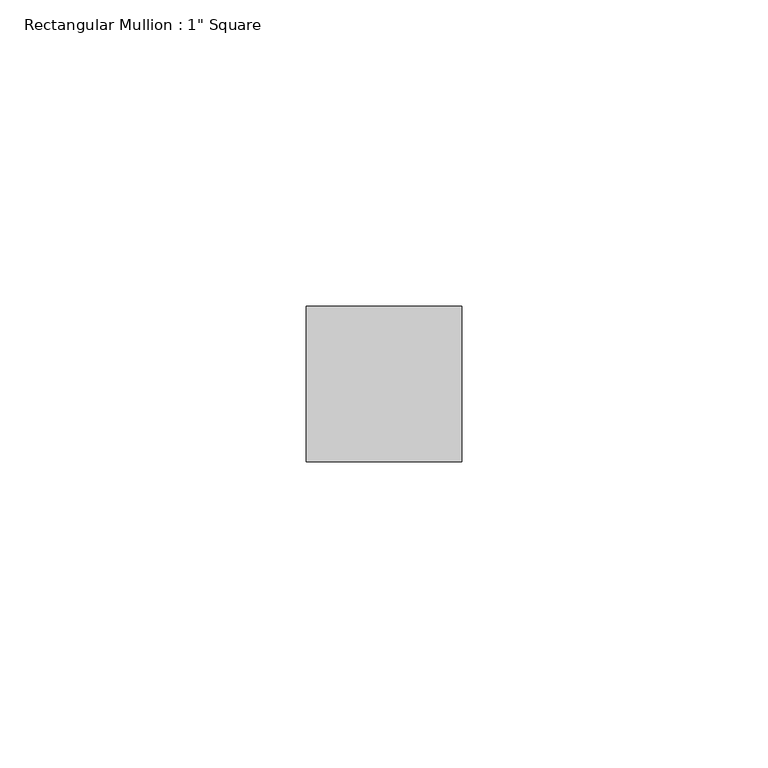
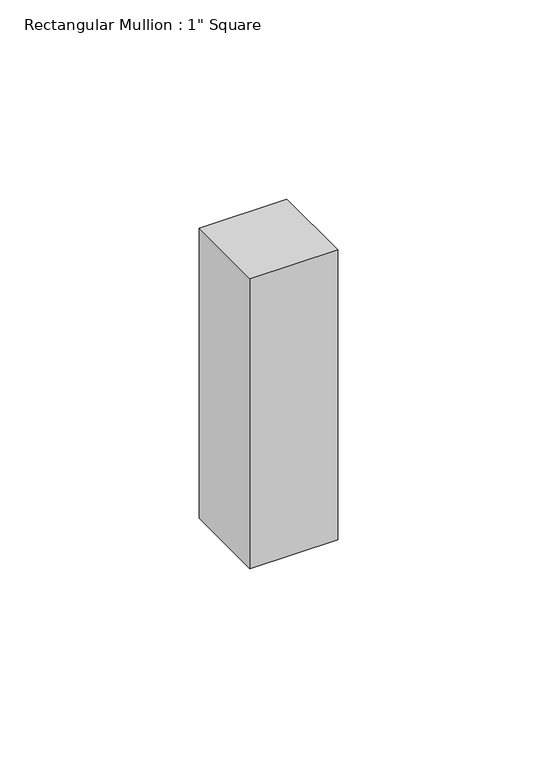
"""IFC4 building model written with IfcOpenShell, lengths in millimetres: member geometry."""

from ifc_helpers import new_model, si_unit, frame, origin, place, context, project, spatial, polyline, outline, extrude, source, transform, mapped, element, save


def member_fbb4b654(model_context):
    return source(origin(), model_context, "Body", "SweptSolid", [
        extrude(outline(polyline([(0.0, 12.7), (0.0, -12.7), (-25.4, -12.7), (-25.4, 12.7), (0.0, 12.7)])), frame((0.0, 0.0, -88.9), z_axis=(0.0, 0.0, 1.0), x_axis=(1.0, 0.0, 0.0)), (0.0, 0.0, 1.0), 88.9),
    ])


if __name__ == "__main__":
    model = new_model("IFC4")
    model_context = context("Model", 3, world=origin())
    ifc_project = project(units=[si_unit("LENGTHUNIT", "METRE", prefix="MILLI")], contexts=[model_context])
    site = spatial("IfcSite", under=ifc_project)
    building = spatial("IfcBuilding", under=site)
    placement = place(None, origin())
    member_shape = member_fbb4b654(model_context)
    element("IfcMember", 1, ObjectType="Rectangular Mullion : 1\" Square", at=placement, inside=building, context=model_context, shape_type="MappedRepresentation", body=[
        mapped(member_shape, transform((0.0, 0.0, 0.0), x_axis=(1.0, 0.0, 0.0), y_axis=(0.0, 1.0, 0.0), z_axis=(0.0, 0.0, 1.0))),
    ])
    save(model, "model.ifc")

# Revit data of these elements
# Type "Rectangular Mullion : 1\" Square"
#   built-in parameter 1007304 = 0.0833333 (stored number, unit not read)
#   built-in parameter 1007301 = 0.0416667 (stored number, unit not read)
#   built-in parameter 1007300 = 0.0416667 (stored number, unit not read)
# Element 1 (IfcMember, "Rectangular Mullion : 1\" Square")
#   Materials on its faces: "black"
# Materials
#   "black": class "Generic", colour RGB 120 120 120, transparency 0, Cost = 0
